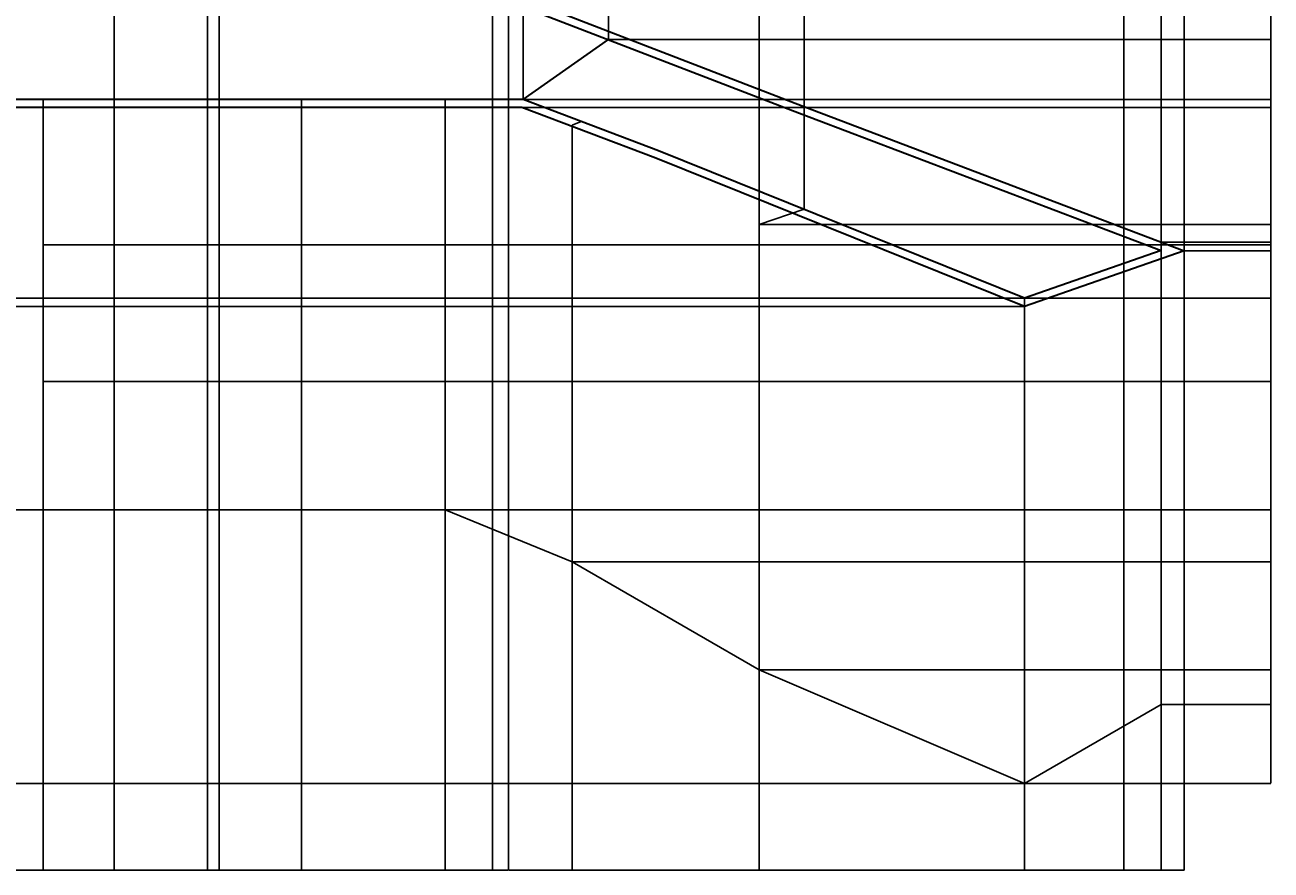
# Model space of a CAD drawing. Units: millimetres. Extents: x 2845 to 7170, y 3531 to 6858.
# Tile 2 of 3: x 4328 to 7170, y 3531 to 5460. Entities that reach past the tile are written whole.
import ezdxf

# ---------------------------------------------------------------- set-up
doc = ezdxf.new("R2010")
doc.units = ezdxf.units.MM
for name, color, linetype, lineweight in [('A-ANNO-DIMS', 2, 'Continuous', 18), ('A-FURN-BASE', 3, 'Continuous', 25), ('A-FURN-CTOP', 6, 'Continuous', 35)]:
    doc.layers.add(name, color=color, linetype=linetype, lineweight=lineweight)
doc.styles.get("Standard").update_dxf_attribs({"font": 'arial.ttf'})
doc.dimstyles.get("Standard").update_dxf_attribs({"dimtxt": 0.18, "dimasz": 0.18, "dimexe": 0.18, "dimexo": 0.0625, "dimgap": 0.09, "dimtad": 0, "dimtih": 1, "dimtoh": 1, "dimdec": 4, "dimzin": 0, "dimdsep": 46, "dimtxsty": 'Standard', "dimcen": 0.09, "dimadec": 0, "dimazin": 0, "dimtfac": 1, "dimtdec": 4, "dimtofl": 0, "dimtmove": 0, "dimatfit": 3, "dimfxl": 1, "dimtolj": 1, "dimtzin": 0, "dimarcsym": 0})

# ---------------------------------------------------------------- blocks, each defined once
blk = doc.blocks.new('*D1')
at = {"layer": 'A-ANNO-DIMS', "color": 0, "lineweight": -2, "transparency": 16777216}
for p, q in [((3042.6, 6659.7), (2844.7, 6659.7)), ((2844.9, 6659.5), (2844.9, 5194.4)), ((2844.9, 3728.9), (2844.9, 5194)), ((6608, 3728.7), (2844.7, 3728.7))]:
    blk.add_line(p, q, dxfattribs=at)
at = {"layer": 'A-ANNO-DIMS', "color": 0, "transparency": 16777216}
for points in [[(2844.9, 6659.5), (2844.9, 6659.5), (2844.9, 6659.7)], [(2844.9, 3728.9), (2844.9, 3728.9), (2844.9, 3728.7)]]:
    blk.add_solid(points, dxfattribs=at)
at = {"layer": 'Defpoints', "color": 0, "transparency": 16777216}
for p in [(2844.9, 6659.7), (3042.7, 6659.7), (6608.1, 3728.7)]:
    blk.add_point(p, dxfattribs=at)
at = {"layer": 'A-ANNO-DIMS', "color": 0, "transparency": 16777216, "insert": (2844.9, 5194.2), "char_height": 0.18, "attachment_point": 5}
blk.add_mtext('\\A1;2931', dxfattribs=at)
blk = doc.blocks.new('*D2')
at = {"layer": 'A-ANNO-DIMS', "color": 0, "lineweight": -2, "transparency": 16777216}
for p, q in [((3042.7, 6659.8), (3042.7, 6857.7)), ((3042.8, 6857.5), (5006.9, 6857.5)), ((6971.9, 6857.5), (5007.8, 6857.5)), ((6972.1, 4944.1), (6972.1, 6857.7))]:
    blk.add_line(p, q, dxfattribs=at)
at = {"layer": 'A-ANNO-DIMS', "color": 0, "transparency": 16777216}
for points in [[(3042.8, 6857.5), (3042.8, 6857.4), (3042.7, 6857.5)], [(6971.9, 6857.5), (6971.9, 6857.4), (6972.1, 6857.5)]]:
    blk.add_solid(points, dxfattribs=at)
at = {"layer": 'Defpoints', "color": 0, "transparency": 16777216}
for p in [(6972.1, 6857.5), (3042.7, 6659.7), (6972.1, 4944.1)]:
    blk.add_point(p, dxfattribs=at)
at = {"layer": 'A-ANNO-DIMS', "color": 0, "transparency": 16777216, "insert": (5007.4, 6857.5), "char_height": 0.18, "attachment_point": 5}
blk.add_mtext('\\A1;3929.4', dxfattribs=at)
blk = doc.blocks.new('*D29')
at = {"layer": 'A-ANNO-DIMS', "color": 0, "lineweight": -2, "transparency": 16777216}
for p, q in [((4531.3, 5812.7), (4531.3, 3530.8)), ((4744.4, 5812.7), (4744.4, 3530.8)), ((4531.4, 3531), (4637.4, 3531)), ((4744.3, 3531), (4638.3, 3531))]:
    blk.add_line(p, q, dxfattribs=at)
at = {"layer": 'A-ANNO-DIMS', "color": 0, "transparency": 16777216}
for points in [[(4531.4, 3531), (4531.4, 3530.9), (4531.3, 3531)], [(4744.3, 3531), (4744.3, 3530.9), (4744.4, 3531)]]:
    blk.add_solid(points, dxfattribs=at)
at = {"layer": 'Defpoints', "color": 0, "transparency": 16777216}
for p in [(4531.3, 5812.8), (4744.4, 5812.8), (4744.4, 3531)]:
    blk.add_point(p, dxfattribs=at)
at = {"layer": 'A-ANNO-DIMS', "color": 0, "transparency": 16777216, "insert": (4637.9, 3531), "char_height": 0.18, "attachment_point": 5}
blk.add_mtext('\\A1;213.17', dxfattribs=at)
blk = doc.blocks.new('*D30')
at = {"layer": 'A-ANNO-DIMS', "color": 0, "lineweight": -2, "transparency": 16777216}
for p, q in [((4744.4, 5812.7), (4744.4, 3530.8)), ((4771.2, 5812.7), (4771.2, 3530.8)), ((4744.6, 3531), (4757.4, 3531)), ((4771, 3531), (4758.3, 3531))]:
    blk.add_line(p, q, dxfattribs=at)
at = {"layer": 'A-ANNO-DIMS', "color": 0, "transparency": 16777216}
for points in [[(4744.6, 3531), (4744.6, 3530.9), (4744.4, 3531)], [(4771, 3531), (4771, 3530.9), (4771.2, 3531)]]:
    blk.add_solid(points, dxfattribs=at)
at = {"layer": 'Defpoints', "color": 0, "transparency": 16777216}
for p in [(4744.4, 5812.8), (4771.2, 5812.8), (4771.2, 3531)]:
    blk.add_point(p, dxfattribs=at)
at = {"layer": 'A-ANNO-DIMS', "color": 0, "transparency": 16777216, "insert": (4757.8, 3531), "char_height": 0.18, "attachment_point": 5}
blk.add_mtext('\\A1;26.776', dxfattribs=at)
blk = doc.blocks.new('*D31')
at = {"layer": 'A-ANNO-DIMS', "color": 0, "lineweight": -2, "transparency": 16777216}
for p, q in [((5394.2, 5812.7), (5394.2, 3530.8)), ((5431.3, 5812.7), (5431.3, 3530.8)), ((5394.4, 3531), (5412.3, 3531)), ((5431.1, 3531), (5413.1, 3531))]:
    blk.add_line(p, q, dxfattribs=at)
at = {"layer": 'A-ANNO-DIMS', "color": 0, "transparency": 16777216}
for points in [[(5394.4, 3531), (5394.4, 3530.9), (5394.2, 3531)], [(5431.1, 3531), (5431.1, 3530.9), (5431.3, 3531)]]:
    blk.add_solid(points, dxfattribs=at)
at = {"layer": 'Defpoints', "color": 0, "transparency": 16777216}
for p in [(5394.2, 5812.8), (5431.3, 5812.8), (5431.3, 3531)]:
    blk.add_point(p, dxfattribs=at)
at = {"layer": 'A-ANNO-DIMS', "color": 0, "transparency": 16777216, "insert": (5412.7, 3531), "char_height": 0.18, "attachment_point": 5}
blk.add_mtext('\\A1;37.06', dxfattribs=at)
blk = doc.blocks.new('*D39')
at = {"layer": 'A-ANNO-DIMS', "color": 0, "lineweight": -2, "transparency": 16777216}
for p, q in [((6834.1, 6135.1), (6834.1, 3530.8)), ((6919.8, 6135.1), (6919.8, 3530.8)), ((6834.3, 3531), (6876.6, 3531)), ((6919.6, 3531), (6877.4, 3531))]:
    blk.add_line(p, q, dxfattribs=at)
at = {"layer": 'A-ANNO-DIMS', "color": 0, "transparency": 16777216}
for points in [[(6834.3, 3531), (6834.3, 3530.9), (6834.1, 3531)], [(6919.6, 3531), (6919.6, 3530.9), (6919.8, 3531)]]:
    blk.add_solid(points, dxfattribs=at)
at = {"layer": 'Defpoints', "color": 0, "transparency": 16777216}
for p in [(6834.1, 6135.2), (6919.8, 6135.2), (6919.8, 3531)]:
    blk.add_point(p, dxfattribs=at)
at = {"layer": 'A-ANNO-DIMS', "color": 0, "transparency": 16777216, "insert": (6877, 3531), "char_height": 0.18, "attachment_point": 5}
blk.add_mtext('\\A1;85.67', dxfattribs=at)
blk = doc.blocks.new('*D40')
at = {"layer": 'A-ANNO-DIMS', "color": 0, "lineweight": -2, "transparency": 16777216}
for p, q in [((3939, 5289.6), (7170, 5289.6)), ((7169.8, 5289.4), (7169.8, 5280.8)), ((3939, 5271.7), (7170, 5271.7)), ((7169.8, 5271.9), (7169.8, 5280.5))]:
    blk.add_line(p, q, dxfattribs=at)
at = {"layer": 'A-ANNO-DIMS', "color": 0, "transparency": 16777216}
for points in [[(7169.8, 5289.4), (7169.8, 5289.4), (7169.8, 5289.6)], [(7169.8, 5271.9), (7169.8, 5271.9), (7169.8, 5271.7)]]:
    blk.add_solid(points, dxfattribs=at)
at = {"layer": 'Defpoints', "color": 0, "transparency": 16777216}
for p in [(3939, 5289.6), (7169.8, 5289.6), (3939, 5271.7)]:
    blk.add_point(p, dxfattribs=at)
at = {"layer": 'A-ANNO-DIMS', "color": 0, "transparency": 16777216, "insert": (7169.8, 5280.6), "char_height": 0.18, "attachment_point": 5}
blk.add_mtext('\\A1;17.853', dxfattribs=at)
blk = doc.blocks.new('*D41')
at = {"layer": 'A-ANNO-DIMS', "color": 0, "lineweight": -2, "transparency": 16777216}
for p, q in [((3939, 5588.8), (7170, 5588.8)), ((7169.8, 5588.6), (7169.8, 5439.4)), ((7169.8, 5289.7), (7169.8, 5439)), ((3939, 5289.6), (7170, 5289.6))]:
    blk.add_line(p, q, dxfattribs=at)
at = {"layer": 'A-ANNO-DIMS', "color": 0, "transparency": 16777216}
for points in [[(7169.8, 5588.6), (7169.8, 5588.6), (7169.8, 5588.8)], [(7169.8, 5289.7), (7169.8, 5289.7), (7169.8, 5289.6)]]:
    blk.add_solid(points, dxfattribs=at)
at = {"layer": 'Defpoints', "color": 0, "transparency": 16777216}
for p in [(3939, 5588.8), (7169.8, 5588.8), (3939, 5289.6)]:
    blk.add_point(p, dxfattribs=at)
at = {"layer": 'A-ANNO-DIMS', "color": 0, "transparency": 16777216, "insert": (7169.8, 5439.2), "char_height": 0.18, "attachment_point": 5}
blk.add_mtext('\\A1;299.2', dxfattribs=at)
blk = doc.blocks.new('*D44')
at = {"layer": 'A-ANNO-DIMS', "color": 0, "lineweight": -2, "transparency": 16777216}
for p, q in [((3939, 5289.6), (3939, 6857.7)), ((3939.1, 6857.5), (4701.3, 6857.5)), ((5464.4, 6857.5), (4702.2, 6857.5)), ((5464.6, 5289.6), (5464.6, 6857.7))]:
    blk.add_line(p, q, dxfattribs=at)
at = {"layer": 'A-ANNO-DIMS', "color": 0, "transparency": 16777216}
for points in [[(3939.1, 6857.5), (3939.1, 6857.4), (3939, 6857.5)], [(5464.4, 6857.5), (5464.4, 6857.4), (5464.6, 6857.5)]]:
    blk.add_solid(points, dxfattribs=at)
at = {"layer": 'Defpoints', "color": 0, "transparency": 16777216}
for p in [(5464.6, 6857.5), (3939, 5289.6), (5464.6, 5289.6)]:
    blk.add_point(p, dxfattribs=at)
at = {"layer": 'A-ANNO-DIMS', "color": 0, "transparency": 16777216, "insert": (4701.8, 6857.5), "char_height": 0.18, "attachment_point": 5}
blk.add_mtext('\\A1;1525.6', dxfattribs=at)
blk = doc.blocks.new('*D45')
at = {"layer": 'A-ANNO-DIMS', "color": 0, "lineweight": -2, "transparency": 16777216}
for p, q in [((5464.6, 5289.6), (5464.6, 6857.7)), ((5464.8, 6857.5), (5561.2, 6857.5)), ((5658.6, 6857.5), (5562.1, 6857.5)), ((5658.7, 5426.7), (5658.7, 6857.7))]:
    blk.add_line(p, q, dxfattribs=at)
at = {"layer": 'A-ANNO-DIMS', "color": 0, "transparency": 16777216}
for points in [[(5464.8, 6857.5), (5464.8, 6857.4), (5464.6, 6857.5)], [(5658.6, 6857.5), (5658.6, 6857.4), (5658.7, 6857.5)]]:
    blk.add_solid(points, dxfattribs=at)
at = {"layer": 'Defpoints', "color": 0, "transparency": 16777216}
for p in [(5658.7, 6857.5), (5658.7, 5426.7), (5464.6, 5289.6)]:
    blk.add_point(p, dxfattribs=at)
at = {"layer": 'A-ANNO-DIMS', "color": 0, "transparency": 16777216, "insert": (5561.7, 6857.5), "char_height": 0.18, "attachment_point": 5}
blk.add_mtext('\\A1;194.16', dxfattribs=at)
blk = doc.blocks.new('*D46')
at = {"layer": 'A-ANNO-DIMS', "color": 0, "lineweight": -2, "transparency": 16777216}
for p, q in [((5658.8, 5426.7), (7170, 5426.7)), ((7169.8, 5426.5), (7169.8, 5358.3)), ((7169.8, 5289.7), (7169.8, 5357.9)), ((5464.6, 5289.6), (7170, 5289.6))]:
    blk.add_line(p, q, dxfattribs=at)
at = {"layer": 'A-ANNO-DIMS', "color": 0, "transparency": 16777216}
for points in [[(7169.8, 5426.5), (7169.8, 5426.5), (7169.8, 5426.7)], [(7169.8, 5289.7), (7169.8, 5289.7), (7169.8, 5289.6)]]:
    blk.add_solid(points, dxfattribs=at)
at = {"layer": 'Defpoints', "color": 0, "transparency": 16777216}
for p in [(5658.7, 5426.7), (7169.8, 5426.7), (5464.6, 5289.6)]:
    blk.add_point(p, dxfattribs=at)
at = {"layer": 'A-ANNO-DIMS', "color": 0, "transparency": 16777216, "insert": (7169.8, 5358.1), "char_height": 0.18, "attachment_point": 5}
blk.add_mtext('\\A1;137.1', dxfattribs=at)
blk = doc.blocks.new('*D47')
at = {"layer": 'A-ANNO-DIMS', "color": 0, "lineweight": -2, "transparency": 16777216}
for p, q in [((6607.5, 4817.5), (2844.7, 4817.5)), ((2844.9, 4817.4), (2844.9, 4273.3)), ((2844.9, 3728.9), (2844.9, 4272.9)), ((6608, 3728.7), (2844.7, 3728.7))]:
    blk.add_line(p, q, dxfattribs=at)
at = {"layer": 'A-ANNO-DIMS', "color": 0, "transparency": 16777216}
for points in [[(2844.9, 4817.4), (2844.9, 4817.4), (2844.9, 4817.5)], [(2844.9, 3728.9), (2844.9, 3728.9), (2844.9, 3728.7)]]:
    blk.add_solid(points, dxfattribs=at)
at = {"layer": 'Defpoints', "color": 0, "transparency": 16777216}
for p in [(2844.9, 4817.5), (6607.6, 4817.5), (6608.1, 3728.7)]:
    blk.add_point(p, dxfattribs=at)
at = {"layer": 'A-ANNO-DIMS', "color": 0, "transparency": 16777216, "insert": (2844.9, 4273.1), "char_height": 0.18, "attachment_point": 5}
blk.add_mtext('\\A1;1088.8', dxfattribs=at)
blk = doc.blocks.new('*D48')
at = {"layer": 'A-ANNO-DIMS', "color": 0, "lineweight": -2, "transparency": 16777216}
for p, q in [((6608, 4836.6), (2844.7, 4836.6)), ((2844.9, 4836.4), (2844.9, 4827.2)), ((6607.5, 4817.5), (2844.7, 4817.5)), ((2844.9, 4817.7), (2844.9, 4826.9))]:
    blk.add_line(p, q, dxfattribs=at)
at = {"layer": 'A-ANNO-DIMS', "color": 0, "transparency": 16777216}
for points in [[(2844.9, 4836.4), (2844.9, 4836.4), (2844.9, 4836.6)], [(2844.9, 4817.7), (2844.9, 4817.7), (2844.9, 4817.5)]]:
    blk.add_solid(points, dxfattribs=at)
at = {"layer": 'Defpoints', "color": 0, "transparency": 16777216}
for p in [(2844.9, 4836.6), (6608.1, 4836.6), (6607.6, 4817.5)]:
    blk.add_point(p, dxfattribs=at)
at = {"layer": 'A-ANNO-DIMS', "color": 0, "transparency": 16777216, "insert": (2844.9, 4827.1), "char_height": 0.18, "attachment_point": 5}
blk.add_mtext('\\A1;19.06', dxfattribs=at)
blk = doc.blocks.new('*D49')
at = {"layer": 'A-ANNO-DIMS', "color": 0, "lineweight": -2, "transparency": 16777216}
for p, q in [((6972.1, 4944.1), (7170, 4944.1)), ((7169.8, 4943.9), (7169.8, 4890.5)), ((7169.8, 4836.8), (7169.8, 4890.2)), ((6608.1, 4836.6), (7170, 4836.6))]:
    blk.add_line(p, q, dxfattribs=at)
at = {"layer": 'A-ANNO-DIMS', "color": 0, "transparency": 16777216}
for points in [[(7169.8, 4943.9), (7169.8, 4943.9), (7169.8, 4944.1)], [(7169.8, 4836.8), (7169.8, 4836.8), (7169.8, 4836.6)]]:
    blk.add_solid(points, dxfattribs=at)
at = {"layer": 'Defpoints', "color": 0, "transparency": 16777216}
for p in [(6972.1, 4944.1), (7169.8, 4944.1), (6608.1, 4836.6)]:
    blk.add_point(p, dxfattribs=at)
at = {"layer": 'A-ANNO-DIMS', "color": 0, "transparency": 16777216, "insert": (7169.8, 4890.3), "char_height": 0.18, "attachment_point": 5}
blk.add_mtext('\\A1;107.48', dxfattribs=at)
blk = doc.blocks.new('*D50')
at = {"layer": 'A-ANNO-DIMS', "color": 0, "lineweight": -2, "transparency": 16777216}
for p, q in [((6972.1, 4944), (6972.1, 3530.8)), ((6607.6, 4817.5), (6607.6, 3530.8)), ((6607.8, 3531), (6789.4, 3531)), ((6971.9, 3531), (6790.3, 3531))]:
    blk.add_line(p, q, dxfattribs=at)
at = {"layer": 'A-ANNO-DIMS', "color": 0, "transparency": 16777216}
for points in [[(6607.8, 3531), (6607.8, 3530.9), (6607.6, 3531)], [(6971.9, 3531), (6971.9, 3530.9), (6972.1, 3531)]]:
    blk.add_solid(points, dxfattribs=at)
at = {"layer": 'Defpoints', "color": 0, "transparency": 16777216}
for p in [(6972.1, 4944.1), (6607.6, 4817.5), (6972.1, 3531)]:
    blk.add_point(p, dxfattribs=at)
at = {"layer": 'A-ANNO-DIMS', "color": 0, "transparency": 16777216, "insert": (6789.8, 3531), "char_height": 0.18, "attachment_point": 5}
blk.add_mtext('\\A1;364.46', dxfattribs=at)
blk = doc.blocks.new('*D51')
at = {"layer": 'A-ANNO-DIMS', "color": 0, "lineweight": -2, "transparency": 16777216}
for p, q in [((6919.9, 4963.9), (7170, 4963.9)), ((7169.8, 4963.8), (7169.8, 4436.5)), ((7169.8, 3908.9), (7169.8, 4436.1)), ((6919.9, 3908.7), (7170, 3908.7))]:
    blk.add_line(p, q, dxfattribs=at)
at = {"layer": 'A-ANNO-DIMS', "color": 0, "transparency": 16777216}
for points in [[(7169.8, 4963.8), (7169.8, 4963.8), (7169.8, 4963.9)], [(7169.8, 3908.9), (7169.8, 3908.9), (7169.8, 3908.7)]]:
    blk.add_solid(points, dxfattribs=at)
at = {"layer": 'Defpoints', "color": 0, "transparency": 16777216}
for p in [(6919.8, 4963.9), (7169.8, 4963.9), (6919.8, 3908.7)]:
    blk.add_point(p, dxfattribs=at)
at = {"layer": 'A-ANNO-DIMS', "color": 0, "transparency": 16777216, "insert": (7169.8, 4436.3), "char_height": 0.18, "attachment_point": 5}
blk.add_mtext('\\A1;1055.2', dxfattribs=at)
blk = doc.blocks.new('*D53')
at = {"layer": 'A-ANNO-DIMS', "color": 0, "lineweight": -2, "transparency": 16777216}
for p, q in [((3939, 4352.7), (3939, 3530.8)), ((4369.7, 4352.7), (4369.7, 3530.8)), ((3939.1, 3531), (4153.9, 3531)), ((4369.5, 3531), (4154.7, 3531))]:
    blk.add_line(p, q, dxfattribs=at)
at = {"layer": 'A-ANNO-DIMS', "color": 0, "transparency": 16777216}
for points in [[(3939.1, 3531), (3939.1, 3530.9), (3939, 3531)], [(4369.5, 3531), (4369.5, 3530.9), (4369.7, 3531)]]:
    blk.add_solid(points, dxfattribs=at)
at = {"layer": 'Defpoints', "color": 0, "transparency": 16777216}
for p in [(3939, 4352.8), (4369.7, 4352.8), (4369.7, 3531)]:
    blk.add_point(p, dxfattribs=at)
at = {"layer": 'A-ANNO-DIMS', "color": 0, "transparency": 16777216, "insert": (4154.3, 3531), "char_height": 0.18, "attachment_point": 5}
blk.add_mtext('\\A1;430.7', dxfattribs=at)
blk = doc.blocks.new('*D54')
at = {"layer": 'A-ANNO-DIMS', "color": 0, "lineweight": -2, "transparency": 16777216}
for p, q in [((4369.7, 4352.7), (4369.7, 3530.8)), ((4958.6, 4352.7), (4958.6, 3530.8)), ((4369.9, 3531), (4663.8, 3531)), ((4958.4, 3531), (4664.5, 3531))]:
    blk.add_line(p, q, dxfattribs=at)
at = {"layer": 'A-ANNO-DIMS', "color": 0, "transparency": 16777216}
for points in [[(4369.9, 3531), (4369.9, 3530.9), (4369.7, 3531)], [(4958.4, 3531), (4958.4, 3530.9), (4958.6, 3531)]]:
    blk.add_solid(points, dxfattribs=at)
at = {"layer": 'Defpoints', "color": 0, "transparency": 16777216}
for p in [(4369.7, 4352.8), (4958.6, 4352.8), (4958.6, 3531)]:
    blk.add_point(p, dxfattribs=at)
at = {"layer": 'A-ANNO-DIMS', "color": 0, "transparency": 16777216, "insert": (4664.1, 3531), "char_height": 0.18, "attachment_point": 5}
blk.add_mtext('\\A1;588.9', dxfattribs=at)
blk = doc.blocks.new('*D55')
at = {"layer": 'A-ANNO-DIMS', "color": 0, "lineweight": -2, "transparency": 16777216}
for p, q in [((4958.6, 4352.7), (4958.6, 3530.8)), ((5286.8, 4352.7), (5286.8, 3530.8)), ((4958.8, 3531), (5122.3, 3531)), ((5286.6, 3531), (5123.1, 3531))]:
    blk.add_line(p, q, dxfattribs=at)
at = {"layer": 'A-ANNO-DIMS', "color": 0, "transparency": 16777216}
for points in [[(4958.8, 3531), (4958.8, 3530.9), (4958.6, 3531)], [(5286.6, 3531), (5286.6, 3530.9), (5286.8, 3531)]]:
    blk.add_solid(points, dxfattribs=at)
at = {"layer": 'Defpoints', "color": 0, "transparency": 16777216}
for p in [(4958.6, 4352.8), (5286.8, 4352.8), (5286.8, 3531)]:
    blk.add_point(p, dxfattribs=at)
at = {"layer": 'A-ANNO-DIMS', "color": 0, "transparency": 16777216, "insert": (5122.7, 3531), "char_height": 0.18, "attachment_point": 5}
blk.add_mtext('\\A1;328.2', dxfattribs=at)
blk = doc.blocks.new('*D56')
at = {"layer": 'A-ANNO-DIMS', "color": 0, "lineweight": -2, "transparency": 16777216}
for p, q in [((5286.8, 4352.7), (5286.8, 3530.8)), ((5576.4, 4234.2), (5576.4, 3530.8)), ((5287, 3531), (5431.1, 3531)), ((5576.2, 3531), (5432.1, 3531))]:
    blk.add_line(p, q, dxfattribs=at)
at = {"layer": 'A-ANNO-DIMS', "color": 0, "transparency": 16777216}
for points in [[(5287, 3531), (5287, 3530.9), (5286.8, 3531)], [(5576.2, 3531), (5576.2, 3530.9), (5576.4, 3531)]]:
    blk.add_solid(points, dxfattribs=at)
at = {"layer": 'Defpoints', "color": 0, "transparency": 16777216}
for p in [(5286.8, 4352.8), (5576.4, 4234.2), (5576.4, 3531)]:
    blk.add_point(p, dxfattribs=at)
at = {"layer": 'A-ANNO-DIMS', "color": 0, "transparency": 16777216, "insert": (5431.6, 3531), "char_height": 0.18, "attachment_point": 5}
blk.add_mtext('\\A1;289.55', dxfattribs=at)
blk = doc.blocks.new('*D57')
at = {"layer": 'A-ANNO-DIMS', "color": 0, "lineweight": -2, "transparency": 16777216}
for p, q in [((5576.4, 4234.2), (5576.4, 3530.8)), ((6003, 3987.8), (6003, 3530.8)), ((5576.5, 3531), (5789.3, 3531)), ((6002.8, 3531), (5790.1, 3531))]:
    blk.add_line(p, q, dxfattribs=at)
at = {"layer": 'A-ANNO-DIMS', "color": 0, "transparency": 16777216}
for points in [[(5576.5, 3531), (5576.5, 3530.9), (5576.4, 3531)], [(6002.8, 3531), (6002.8, 3530.9), (6003, 3531)]]:
    blk.add_solid(points, dxfattribs=at)
at = {"layer": 'Defpoints', "color": 0, "transparency": 16777216}
for p in [(5576.4, 4234.2), (6003, 3987.9), (6003, 3531)]:
    blk.add_point(p, dxfattribs=at)
at = {"layer": 'A-ANNO-DIMS', "color": 0, "transparency": 16777216, "insert": (5789.7, 3531), "char_height": 0.18, "attachment_point": 5}
blk.add_mtext('\\A1;426.7', dxfattribs=at)
blk = doc.blocks.new('*D58')
at = {"layer": 'A-ANNO-DIMS', "color": 0, "lineweight": -2, "transparency": 16777216}
for p, q in [((6003, 3987.8), (6003, 3530.8)), ((6608.1, 3728.7), (6608.1, 3530.8)), ((6003.2, 3531), (6305.3, 3531)), ((6607.9, 3531), (6305.8, 3531))]:
    blk.add_line(p, q, dxfattribs=at)
at = {"layer": 'A-ANNO-DIMS', "color": 0, "transparency": 16777216}
for points in [[(6003.2, 3531), (6003.2, 3530.9), (6003, 3531)], [(6607.9, 3531), (6607.9, 3530.9), (6608.1, 3531)]]:
    blk.add_solid(points, dxfattribs=at)
at = {"layer": 'Defpoints', "color": 0, "transparency": 16777216}
for p in [(6003, 3987.9), (6608.1, 3728.7), (6608.1, 3531)]:
    blk.add_point(p, dxfattribs=at)
at = {"layer": 'A-ANNO-DIMS', "color": 0, "transparency": 16777216, "insert": (6305.5, 3531), "char_height": 0.18, "attachment_point": 5}
blk.add_mtext('\\A1;605', dxfattribs=at)
blk = doc.blocks.new('*D59')
at = {"layer": 'A-ANNO-DIMS', "color": 0, "lineweight": -2, "transparency": 16777216}
for p, q in [((6919.8, 3908.6), (6919.8, 3530.8)), ((6608.1, 3728.7), (6608.1, 3530.8)), ((6608.3, 3531), (6763.5, 3531)), ((6919.6, 3531), (6764.4, 3531))]:
    blk.add_line(p, q, dxfattribs=at)
at = {"layer": 'A-ANNO-DIMS', "color": 0, "transparency": 16777216}
for points in [[(6608.3, 3531), (6608.3, 3530.9), (6608.1, 3531)], [(6919.6, 3531), (6919.6, 3530.9), (6919.8, 3531)]]:
    blk.add_solid(points, dxfattribs=at)
at = {"layer": 'Defpoints', "color": 0, "transparency": 16777216}
for p in [(6919.8, 3908.7), (6608.1, 3728.7), (6919.8, 3531)]:
    blk.add_point(p, dxfattribs=at)
at = {"layer": 'A-ANNO-DIMS', "color": 0, "transparency": 16777216, "insert": (6763.9, 3531), "char_height": 0.18, "attachment_point": 5}
blk.add_mtext('\\A1;311.74', dxfattribs=at)
blk = doc.blocks.new('*D60')
at = {"layer": 'A-ANNO-DIMS', "color": 0, "lineweight": -2, "transparency": 16777216}
for p, q in [((5286.9, 5289.6), (7170, 5289.6)), ((7169.8, 5289.4), (7169.8, 4821.3)), ((7169.8, 4352.9), (7169.8, 4821)), ((5286.9, 4352.8), (7170, 4352.8))]:
    blk.add_line(p, q, dxfattribs=at)
at = {"layer": 'A-ANNO-DIMS', "color": 0, "transparency": 16777216}
for points in [[(7169.8, 5289.4), (7169.8, 5289.4), (7169.8, 5289.6)], [(7169.8, 4352.9), (7169.8, 4352.9), (7169.8, 4352.8)]]:
    blk.add_solid(points, dxfattribs=at)
at = {"layer": 'Defpoints', "color": 0, "transparency": 16777216}
for p in [(5286.8, 5289.6), (7169.8, 5289.6), (5286.8, 4352.8)]:
    blk.add_point(p, dxfattribs=at)
at = {"layer": 'A-ANNO-DIMS', "color": 0, "transparency": 16777216, "insert": (7169.8, 4821.2), "char_height": 0.18, "attachment_point": 5}
blk.add_mtext('\\A1;936.8', dxfattribs=at)
blk = doc.blocks.new('*D61')
at = {"layer": 'A-ANNO-DIMS', "color": 0, "lineweight": -2, "transparency": 16777216}
for p, q in [((4369.7, 4646.3), (7170, 4646.3)), ((7169.8, 4646.2), (7169.8, 4499.7)), ((7169.8, 4352.9), (7169.8, 4499.4)), ((4369.7, 4352.8), (7170, 4352.8))]:
    blk.add_line(p, q, dxfattribs=at)
at = {"layer": 'A-ANNO-DIMS', "color": 0, "transparency": 16777216}
for points in [[(7169.8, 4646.2), (7169.8, 4646.2), (7169.8, 4646.3)], [(7169.8, 4352.9), (7169.8, 4352.9), (7169.8, 4352.8)]]:
    blk.add_solid(points, dxfattribs=at)
at = {"layer": 'Defpoints', "color": 0, "transparency": 16777216}
for p in [(4369.7, 4646.3), (7169.8, 4646.3), (4369.7, 4352.8)]:
    blk.add_point(p, dxfattribs=at)
at = {"layer": 'A-ANNO-DIMS', "color": 0, "transparency": 16777216, "insert": (7169.8, 4499.5), "char_height": 0.18, "attachment_point": 5}
blk.add_mtext('\\A1;293.6', dxfattribs=at)
blk = doc.blocks.new('*D62')
at = {"layer": 'A-ANNO-DIMS', "color": 0, "lineweight": -2, "transparency": 16777216}
for p, q in [((4369.7, 4957.9), (7170, 4957.9)), ((7169.8, 4957.7), (7169.8, 4802.3)), ((7169.8, 4646.5), (7169.8, 4801.9)), ((4369.7, 4646.3), (7170, 4646.3))]:
    blk.add_line(p, q, dxfattribs=at)
at = {"layer": 'A-ANNO-DIMS', "color": 0, "transparency": 16777216}
for points in [[(7169.8, 4957.7), (7169.8, 4957.7), (7169.8, 4957.9)], [(7169.8, 4646.5), (7169.8, 4646.5), (7169.8, 4646.3)]]:
    blk.add_solid(points, dxfattribs=at)
at = {"layer": 'Defpoints', "color": 0, "transparency": 16777216}
for p in [(4369.7, 4957.9), (7169.8, 4957.9), (4369.7, 4646.3)]:
    blk.add_point(p, dxfattribs=at)
at = {"layer": 'A-ANNO-DIMS', "color": 0, "transparency": 16777216, "insert": (7169.8, 4802.1), "char_height": 0.18, "attachment_point": 5}
blk.add_mtext('\\A1;311.6', dxfattribs=at)
blk = doc.blocks.new('*D63')
at = {"layer": 'A-ANNO-DIMS', "color": 0, "lineweight": -2, "transparency": 16777216}
for p, q in [((4369.7, 5289.6), (7170, 5289.6)), ((7169.8, 5289.4), (7169.8, 5123.9)), ((7169.8, 4958.1), (7169.8, 5123.6)), ((4369.7, 4957.9), (7170, 4957.9))]:
    blk.add_line(p, q, dxfattribs=at)
at = {"layer": 'A-ANNO-DIMS', "color": 0, "transparency": 16777216}
for points in [[(7169.8, 5289.4), (7169.8, 5289.4), (7169.8, 5289.6)], [(7169.8, 4958.1), (7169.8, 4958.1), (7169.8, 4957.9)]]:
    blk.add_solid(points, dxfattribs=at)
at = {"layer": 'Defpoints', "color": 0, "transparency": 16777216}
for p in [(4369.7, 5289.6), (7169.8, 5289.6), (4369.7, 4957.9)]:
    blk.add_point(p, dxfattribs=at)
at = {"layer": 'A-ANNO-DIMS', "color": 0, "transparency": 16777216, "insert": (7169.8, 5123.7), "char_height": 0.18, "attachment_point": 5}
blk.add_mtext('\\A1;331.64', dxfattribs=at)
blk = doc.blocks.new('*D64')
at = {"layer": 'A-ANNO-DIMS', "color": 0, "lineweight": -2, "transparency": 16777216}
for p, q in [((5286.9, 4352.8), (7170, 4352.8)), ((7169.8, 4352.6), (7169.8, 4293.7)), ((7169.8, 4234.4), (7169.8, 4293.3)), ((5576.4, 4234.2), (7170, 4234.2))]:
    blk.add_line(p, q, dxfattribs=at)
at = {"layer": 'A-ANNO-DIMS', "color": 0, "transparency": 16777216}
for points in [[(7169.8, 4352.6), (7169.8, 4352.6), (7169.8, 4352.8)], [(7169.8, 4234.4), (7169.8, 4234.4), (7169.8, 4234.2)]]:
    blk.add_solid(points, dxfattribs=at)
at = {"layer": 'Defpoints', "color": 0, "transparency": 16777216}
for p in [(5286.8, 4352.8), (5576.4, 4234.2), (7169.8, 4234.2)]:
    blk.add_point(p, dxfattribs=at)
at = {"layer": 'A-ANNO-DIMS', "color": 0, "transparency": 16777216, "insert": (7169.8, 4293.5), "char_height": 0.18, "attachment_point": 5}
blk.add_mtext('\\A1;118.53', dxfattribs=at)
blk = doc.blocks.new('*D65')
at = {"layer": 'A-ANNO-DIMS', "color": 0, "lineweight": -2, "transparency": 16777216}
for p, q in [((5576.4, 4234.2), (7170, 4234.2)), ((7169.8, 4234), (7169.8, 4111.2)), ((7169.8, 3988.1), (7169.8, 4110.9)), ((6003.1, 3987.9), (7170, 3987.9))]:
    blk.add_line(p, q, dxfattribs=at)
at = {"layer": 'A-ANNO-DIMS', "color": 0, "transparency": 16777216}
for points in [[(7169.8, 4234), (7169.8, 4234), (7169.8, 4234.2)], [(7169.8, 3988.1), (7169.8, 3988.1), (7169.8, 3987.9)]]:
    blk.add_solid(points, dxfattribs=at)
at = {"layer": 'Defpoints', "color": 0, "transparency": 16777216}
for p in [(5576.4, 4234.2), (6003, 3987.9), (7169.8, 3987.9)]:
    blk.add_point(p, dxfattribs=at)
at = {"layer": 'A-ANNO-DIMS', "color": 0, "transparency": 16777216, "insert": (7169.8, 4111.1), "char_height": 0.18, "attachment_point": 5}
blk.add_mtext('\\A1;246.33', dxfattribs=at)
blk = doc.blocks.new('*D66')
at = {"layer": 'A-ANNO-DIMS', "color": 0, "lineweight": -2, "transparency": 16777216}
for p, q in [((6003.1, 3987.9), (7170, 3987.9)), ((7169.8, 3987.7), (7169.8, 3858.5)), ((7169.8, 3728.9), (7169.8, 3858.1)), ((6608.1, 3728.7), (7170, 3728.7))]:
    blk.add_line(p, q, dxfattribs=at)
at = {"layer": 'A-ANNO-DIMS', "color": 0, "transparency": 16777216}
for points in [[(7169.8, 3987.7), (7169.8, 3987.7), (7169.8, 3987.9)], [(7169.8, 3728.9), (7169.8, 3728.9), (7169.8, 3728.7)]]:
    blk.add_solid(points, dxfattribs=at)
at = {"layer": 'Defpoints', "color": 0, "transparency": 16777216}
for p in [(6003, 3987.9), (6608.1, 3728.7), (7169.8, 3728.7)]:
    blk.add_point(p, dxfattribs=at)
at = {"layer": 'A-ANNO-DIMS', "color": 0, "transparency": 16777216, "insert": (7169.8, 3858.3), "char_height": 0.18, "attachment_point": 5}
blk.add_mtext('\\A1;259.2', dxfattribs=at)
blk = doc.blocks.new('*D67')
at = {"layer": 'A-ANNO-DIMS', "color": 0, "lineweight": -2, "transparency": 16777216}
for p, q in [((6919.9, 3908.7), (7170, 3908.7)), ((7169.8, 3908.5), (7169.8, 3818.9)), ((7169.8, 3728.9), (7169.8, 3818.5)), ((6608.1, 3728.7), (7170, 3728.7))]:
    blk.add_line(p, q, dxfattribs=at)
at = {"layer": 'A-ANNO-DIMS', "color": 0, "transparency": 16777216}
for points in [[(7169.8, 3908.5), (7169.8, 3908.5), (7169.8, 3908.7)], [(7169.8, 3728.9), (7169.8, 3728.9), (7169.8, 3728.7)]]:
    blk.add_solid(points, dxfattribs=at)
at = {"layer": 'Defpoints', "color": 0, "transparency": 16777216}
for p in [(6919.8, 3908.7), (7169.8, 3908.7), (6608.1, 3728.7)]:
    blk.add_point(p, dxfattribs=at)
at = {"layer": 'A-ANNO-DIMS', "color": 0, "transparency": 16777216, "insert": (7169.8, 3818.7), "char_height": 0.18, "attachment_point": 5}
blk.add_mtext('\\A1;180', dxfattribs=at)
blk = doc.blocks.new('*D68')
at = {"layer": 'A-ANNO-DIMS', "color": 0, "lineweight": -2, "transparency": 16777216}
for p, q in [((6003.1, 5004.6), (7170, 5004.6)), ((7169.8, 5004.5), (7169.8, 4496.4)), ((7169.8, 3988.1), (7169.8, 4496.1)), ((6003.1, 3987.9), (7170, 3987.9))]:
    blk.add_line(p, q, dxfattribs=at)
at = {"layer": 'A-ANNO-DIMS', "color": 0, "transparency": 16777216}
for points in [[(7169.8, 5004.5), (7169.8, 5004.5), (7169.8, 5004.6)], [(7169.8, 3988.1), (7169.8, 3988.1), (7169.8, 3987.9)]]:
    blk.add_solid(points, dxfattribs=at)
at = {"layer": 'Defpoints', "color": 0, "transparency": 16777216}
for p in [(6003, 5004.6), (7169.8, 5004.6), (6003, 3987.9)]:
    blk.add_point(p, dxfattribs=at)
at = {"layer": 'A-ANNO-DIMS', "color": 0, "transparency": 16777216, "insert": (7169.8, 4496.3), "char_height": 0.18, "attachment_point": 5}
blk.add_mtext('\\A1;1016.7', dxfattribs=at)
blk = doc.blocks.new('*D69')
at = {"layer": 'A-ANNO-DIMS', "color": 0, "lineweight": -2, "transparency": 16777216}
for p, q in [((6003, 5004.7), (6003, 6857.7)), ((6003.2, 6857.5), (6053.8, 6857.5)), ((6105.3, 6857.5), (6054.7, 6857.5)), ((6105.5, 5039.1), (6105.5, 6857.7))]:
    blk.add_line(p, q, dxfattribs=at)
at = {"layer": 'A-ANNO-DIMS', "color": 0, "transparency": 16777216}
for points in [[(6003.2, 6857.5), (6003.2, 6857.4), (6003, 6857.5)], [(6105.3, 6857.5), (6105.3, 6857.4), (6105.5, 6857.5)]]:
    blk.add_solid(points, dxfattribs=at)
at = {"layer": 'Defpoints', "color": 0, "transparency": 16777216}
for p in [(6105.5, 6857.5), (6105.5, 5039), (6003, 5004.6)]:
    blk.add_point(p, dxfattribs=at)
at = {"layer": 'A-ANNO-DIMS', "color": 0, "transparency": 16777216, "insert": (6054.2, 6857.5), "char_height": 0.18, "attachment_point": 5}
blk.add_mtext('\\A1;102.43', dxfattribs=at)

msp = doc.modelspace()

# ---------------------------------------------------------------- linework, layer by layer
at = {"layer": 'A-FURN-BASE', "extrusion": (0, 0, -1)}
for p, q in [((4369.677, 5289.563), (4369.677, 4352.7588)), ((4958.6146, 5289.563), (4958.6146, 4352.7588)), ((5286.8154, 5289.563), (5286.8154, 4352.7588)), ((5576.362, 5231.1675), (5597.0289, 5239.443)), ((5576.362, 4234.2264), (5576.362, 5231.1675)), ((4369.677, 4957.9249), (4958.6146, 4957.9249)), ((6919.8193, 4944.8329), (6919.8193, 4963.9316)), ((4369.677, 4646.3332), (4958.6146, 4646.3332)), ((4369.677, 4352.7588), (3938.9578, 4352.7588)), ((4958.6146, 4352.7588), (4369.677, 4352.7588)), ((5286.8154, 4352.7588), (4958.6146, 4352.7588)), ((5286.8154, 4352.7588), (5576.362, 4234.2264)), ((5576.362, 4234.2264), (5576.362, 4234.2264))]:
    msp.add_line(p, q, dxfattribs=at)
for points in [[(-5576.362, 4234.2264), (-6003.02, 3987.8952), (-6003.02, 5004.6356), (-6105.4534, 5038.9886)], [(-6608.0753, 4836.5939), (-6608.0753, 3728.7204), (-6919.8193, 3908.7059), (-6919.8193, 4944.8329)], [(-6003.02, 3987.8952), (-6608.0753, 3728.7204), (-6608.0753, 4836.5939)]]:
    msp.add_lwpolyline(points, dxfattribs=at)
at = {"layer": 'A-FURN-CTOP', "extrusion": (0, 0, -1)}
msp.add_line((5464.5775, 5289.563), (5658.7423, 5426.6764), dxfattribs=at)
for points in [[(-3938.9578, 5606.6435), (-5242.2853, 5606.6435), (-6084.9137, 5281.2335), (-6972.0668, 4944.0752), (-6607.6118, 4817.5346), (-5766.7252, 5156.141), (-5461.3127, 5271.7102), (-4164.5775, 5271.7102), (-3938.9578, 5271.7102)], [(-3938.9578, 5588.7906), (-5238.9578, 5588.7906), (-6078.5267, 5264.5621), (-6919.8193, 4944.8329), (-6608.0753, 4836.5939), (-5773.2194, 5172.7719), (-5464.5775, 5289.563), (-4164.5775, 5289.563), (-3938.9578, 5289.563)]]:
    msp.add_lwpolyline(points, dxfattribs=at)

# ---------------------------------------------------------------- dimensions: what is measured, and where the dimension line sits
at = {"layer": 'A-ANNO-DIMS'}
for base, p1, p2, override, picture, middle in [((6972.0668, 6857.4724), (3042.6566, 6659.7224), (6972.0668, 4944.0752), {"dimdec": 1, "dimlfac": 1, "dimrnd": 0, "dimzin": 0, "dimdsep": 46, "dimlunit": 2}, '*D2', (5007.3617, 6857.4724)), ((5464.5775, 6857.4724), (3938.9578, 5289.563), (5464.5775, 5289.563), {"dimdec": 1, "dimlfac": 1, "dimrnd": 0, "dimzin": 0, "dimdsep": 46, "dimlunit": 2}, '*D44', (4701.7677, 6857.4724)), ((5658.7423, 6857.4724), (5464.5775, 5289.563), (5658.7423, 5426.6764), {"dimdec": 2, "dimlfac": 1, "dimrnd": 0, "dimzin": 0, "dimdsep": 46, "dimlunit": 2}, '*D45', (5561.6599, 6857.4724)), ((6105.4534, 6857.4724), (6003.02, 5004.6356), (6105.4534, 5038.9886), {"dimdec": 2, "dimlfac": 1, "dimrnd": 0, "dimzin": 0, "dimdsep": 46, "dimlunit": 2}, '*D69', (6054.2367, 6857.4724)), ((6919.8193, 3530.9704), (6834.145, 6135.1857), (6919.8193, 6135.1857), {"dimdec": 2, "dimlfac": 1, "dimrnd": 0, "dimzin": 0, "dimdsep": 46, "dimlunit": 2}, '*D39', (6876.9821, 3530.9704)), ((4744.4359, 3530.9704), (4531.2682, 5812.7588), (4744.4359, 5812.7588), {"dimdec": 2, "dimlfac": 1, "dimrnd": 0, "dimzin": 0, "dimdsep": 46, "dimlunit": 2}, '*D29', (4637.852, 3530.9704)), ((4771.2123, 3530.9704), (4744.4359, 5812.7588), (4771.2123, 5812.7588), {"dimdec": 3, "dimlfac": 1, "dimrnd": 0, "dimzin": 0, "dimdsep": 46, "dimlunit": 2}, '*D30', (4757.8241, 3530.9704)), ((5431.2682, 3530.9704), (5394.2056, 5812.7588), (5431.2682, 5812.7588), {"dimdec": 2, "dimlfac": 1, "dimrnd": 0, "dimzin": 0, "dimdsep": 46, "dimlunit": 2}, '*D31', (5412.7369, 3530.9704)), ((6972.06684, 3530.97043), (6607.61178, 4817.53463), (6972.06684, 4944.07518), {"dimdec": 2, "dimlfac": 1, "dimrnd": 0, "dimzin": 0, "dimdsep": 46, "dimlunit": 2}, '*D50', (6789.83931, 3530.97043)), ((4369.677, 3530.9704), (3938.9578, 4352.7588), (4369.677, 4352.7588), {"dimdec": 1, "dimlfac": 1, "dimrnd": 0, "dimzin": 0, "dimdsep": 46, "dimlunit": 2}, '*D53', (4154.3174, 3530.9704)), ((4958.6146, 3530.9704), (4369.677, 4352.7588), (4958.6146, 4352.7588), {"dimdec": 1, "dimlfac": 1, "dimrnd": 0, "dimzin": 0, "dimdsep": 46, "dimlunit": 2}, '*D54', (4664.1458, 3530.9704)), ((5286.8154, 3530.9704), (4958.6146, 4352.7588), (5286.8154, 4352.7588), {"dimdec": 1, "dimlfac": 1, "dimrnd": 0, "dimzin": 0, "dimdsep": 46, "dimlunit": 2}, '*D55', (5122.715, 3530.9704)), ((5576.362, 3530.9704), (5286.8154, 4352.7588), (5576.362, 4234.2264), {"dimdec": 2, "dimlfac": 1, "dimrnd": 0, "dimzin": 0, "dimdsep": 46, "dimlunit": 2}, '*D56', (5431.5887, 3530.9704)), ((6003.02, 3530.9704), (5576.362, 4234.2264), (6003.02, 3987.8952), {"dimdec": 1, "dimlfac": 1, "dimrnd": 0, "dimzin": 0, "dimdsep": 46, "dimlunit": 2}, '*D57', (5789.691, 3530.9704)), ((6608.0753, 3530.9704), (6003.02, 3987.8952), (6608.0753, 3728.7204), {"dimdec": 0, "dimlfac": 1, "dimrnd": 0, "dimzin": 0, "dimdsep": 46, "dimlunit": 2}, '*D58', (6305.5476, 3530.9704)), ((6919.8193, 3530.9704), (6608.0753, 3728.7204), (6919.8193, 3908.7059), {"dimdec": 2, "dimlfac": 1, "dimrnd": 0, "dimzin": 0, "dimdsep": 46, "dimlunit": 2}, '*D59', (6763.9473, 3530.9704))]:
    dim = msp.add_linear_dim(base=base, p1=p1, p2=p2, dimstyle='Standard', override=override, dxfattribs=at)
    dim.commit()
    dim.dimension.update_dxf_attribs({"geometry": picture, "text_midpoint": middle})
for base, p1, p2, override, picture, middle in [((2844.9066, 6659.7224), (6608.0753, 3728.7204), (3042.6566, 6659.7224), {"dimdec": 0, "dimlfac": 1, "dimrnd": 0, "dimzin": 0, "dimdsep": 46, "dimlunit": 2}, '*D1', (2844.9066, 5194.2214)), ((7169.8168, 5588.7906), (3938.9578, 5289.563), (3938.9578, 5588.7906), {"dimdec": 1, "dimlfac": 1, "dimrnd": 0, "dimzin": 0, "dimdsep": 46, "dimlunit": 2}, '*D41', (7169.8168, 5439.1768)), ((7169.8168, 5426.6764), (5464.5775, 5289.563), (5658.7423, 5426.6764), {"dimdec": 1, "dimlfac": 1, "dimrnd": 0, "dimzin": 0, "dimdsep": 46, "dimlunit": 2}, '*D46', (7169.8168, 5358.1197)), ((7169.8168, 5289.563), (3938.9578, 5271.7102), (3938.9578, 5289.563), {"dimdec": 3, "dimlfac": 1, "dimrnd": 0, "dimzin": 0, "dimdsep": 46, "dimlunit": 2}, '*D40', (7169.8168, 5280.6366)), ((7169.8168, 5289.563), (4369.677, 4957.9249), (4369.677, 5289.563), {"dimdec": 2, "dimlfac": 1, "dimrnd": 0, "dimzin": 0, "dimdsep": 46, "dimlunit": 2}, '*D63', (7169.8168, 5123.744)), ((7169.8168, 5289.563), (5286.8154, 4352.7588), (5286.8154, 5289.563), {"dimdec": 1, "dimlfac": 1, "dimrnd": 0, "dimzin": 0, "dimdsep": 46, "dimlunit": 2}, '*D60', (7169.8168, 4821.1609)), ((7169.8168, 5004.6356), (6003.02, 3987.8952), (6003.02, 5004.6356), {"dimdec": 1, "dimlfac": 1, "dimrnd": 0, "dimzin": 0, "dimdsep": 46, "dimlunit": 2}, '*D68', (7169.8168, 4496.2654)), ((7169.8168, 4957.9249), (4369.677, 4646.3332), (4369.677, 4957.9249), {"dimdec": 1, "dimlfac": 1, "dimrnd": 0, "dimzin": 0, "dimdsep": 46, "dimlunit": 2}, '*D62', (7169.8168, 4802.1291)), ((7169.8168, 4963.9316), (6919.8193, 3908.7059), (6919.8193, 4963.9316), {"dimdec": 1, "dimlfac": 1, "dimrnd": 0, "dimzin": 0, "dimdsep": 46, "dimlunit": 2}, '*D51', (7169.8168, 4436.3188)), ((7169.8168, 4944.0752), (6608.0753, 4836.5939), (6972.0668, 4944.0752), {"dimdec": 2, "dimlfac": 1, "dimrnd": 0, "dimzin": 0, "dimdsep": 46, "dimlunit": 2}, '*D49', (7169.8168, 4890.3345)), ((2844.9066, 4836.5939), (6607.6118, 4817.5346), (6608.0753, 4836.5939), {"dimdec": 2, "dimlfac": 1, "dimrnd": 0, "dimzin": 0, "dimdsep": 46, "dimlunit": 2}, '*D48', (2844.9066, 4827.0643)), ((2844.9066, 4817.5346), (6608.0753, 3728.7204), (6607.6118, 4817.5346), {"dimdec": 1, "dimlfac": 1, "dimrnd": 0, "dimzin": 0, "dimdsep": 46, "dimlunit": 2}, '*D47', (2844.9066, 4273.1275)), ((7169.8168, 4646.3332), (4369.677, 4352.7588), (4369.677, 4646.3332), {"dimdec": 1, "dimlfac": 1, "dimrnd": 0, "dimzin": 0, "dimdsep": 46, "dimlunit": 2}, '*D61', (7169.8168, 4499.546)), ((7169.8168, 4234.2264), (5286.8154, 4352.7588), (5576.362, 4234.2264), {"dimdec": 2, "dimlfac": 1, "dimrnd": 0, "dimzin": 0, "dimdsep": 46, "dimlunit": 2}, '*D64', (7169.8168, 4293.4926)), ((7169.8168, 3987.8952), (5576.362, 4234.2264), (6003.02, 3987.8952), {"dimdec": 2, "dimlfac": 1, "dimrnd": 0, "dimzin": 0, "dimdsep": 46, "dimlunit": 2}, '*D65', (7169.8168, 4111.0608)), ((7169.8168, 3728.7204), (6003.02, 3987.8952), (6608.0753, 3728.7204), {"dimdec": 1, "dimlfac": 1, "dimrnd": 0, "dimzin": 0, "dimdsep": 46, "dimlunit": 2}, '*D66', (7169.8168, 3858.3078)), ((7169.8168, 3908.7059), (6608.0753, 3728.7204), (6919.8193, 3908.7059), {"dimdec": 0, "dimlfac": 1, "dimrnd": 0, "dimzin": 0, "dimdsep": 46, "dimlunit": 2}, '*D67', (7169.8168, 3818.7132))]:
    dim = msp.add_linear_dim(base=base, p1=p1, p2=p2, angle=90, dimstyle='Standard', override=override, dxfattribs=at)
    dim.commit()
    dim.dimension.update_dxf_attribs({"geometry": picture, "text_midpoint": middle})

doc.saveas('drawing.dxf')
